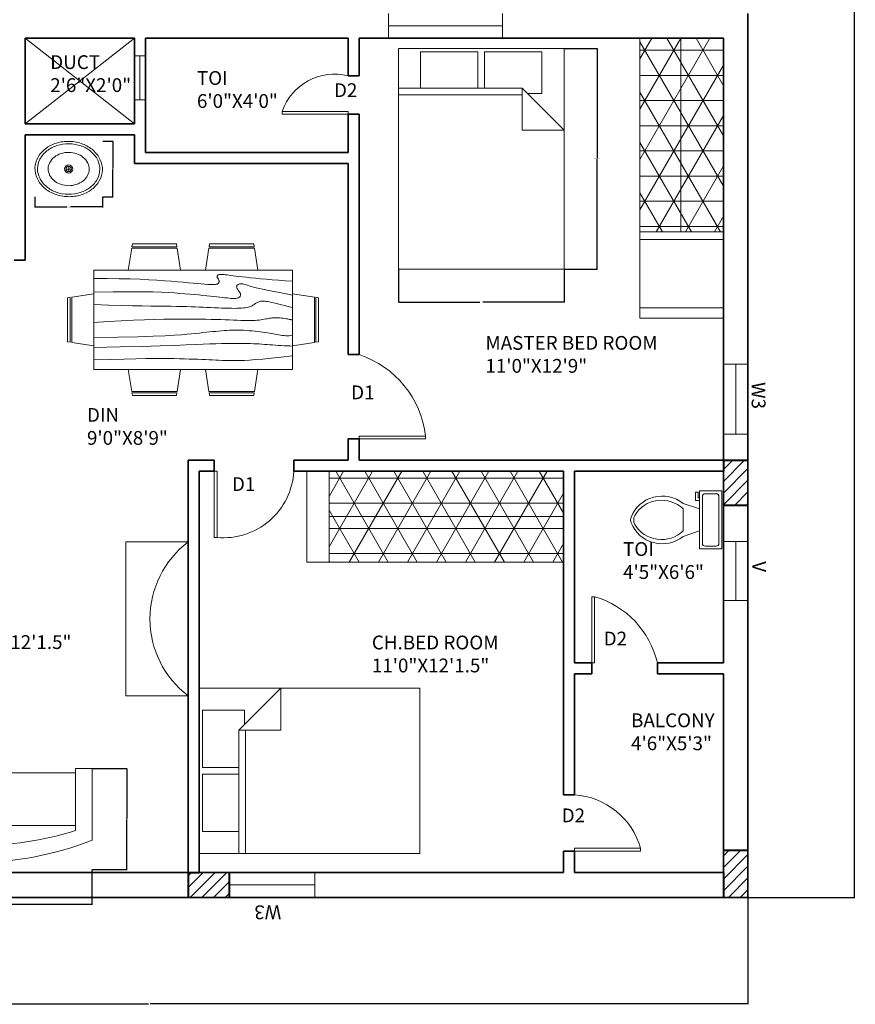
# Model space of a CAD drawing. Units: inches. Extents: x -86 to 2463, y -1058 to 68.
# Tile 2 of 17: x 123 to 426, y -740 to -383. Entities that reach past the tile are written whole.
import ezdxf

# ---------------------------------------------------------------- set-up
doc = ezdxf.new("R2010")
doc.units = ezdxf.units.IN
doc.header["$MEASUREMENT"] = 0
for name, color, linetype, lineweight in [('A-ANNO-DIMS', 2, 'Continuous', 18), ('A-ANNO-TEXT', 7, 'Continuous', 18), ('A-AREA-IDEN', 7, 'Continuous', 18), ('A-COLS', 7, 'Continuous', 40), ('A-COLS-PATT', 252, 'Continuous', 13), ('A-DOOR', 3, 'Continuous', 18), ('A-FLOR-CASE', 8, 'Continuous', 18), ('A-FLOR-CASE-PATT', 252, 'Continuous', 13), ('A-FLOR-FIXT', 9, 'Continuous', 18), ('A-FLOR-OPEN', 8, 'Continuous', 13), ('A-FURN', 8, 'Continuous', 18), ('A-GLAZ', 4, 'Continuous', 18), ('A-WALL', 7, 'Continuous', 35)]:
    doc.layers.add(name, color=color, linetype=linetype, lineweight=lineweight)
doc.styles.get("Standard").update_dxf_attribs({"font": 'arial.ttf'})
doc.dimstyles.get("Standard").update_dxf_attribs({"dimtxt": 0.18, "dimasz": 0.18, "dimexe": 0.18, "dimexo": 0.0625, "dimgap": 0.09, "dimtad": 0, "dimtih": 1, "dimtoh": 1, "dimdec": 4, "dimzin": 0, "dimdsep": 46, "dimtxsty": 'Standard', "dimcen": 0.09, "dimadec": 0, "dimazin": 0, "dimtfac": 1, "dimtdec": 4, "dimtofl": 0, "dimtmove": 0, "dimatfit": 3, "dimfxl": 1, "dimtolj": 1, "dimtzin": 0, "dimarcsym": 0})
pattern_1 = [(45, (-1015.1314, -586.0864), (-2.1213203, 2.1213203), [])]
pattern_2 = [(0, (-1015.131, -586.086), (0, 9.125), []), (60, (-1015.131, -586.086), (-7.90248, 4.5625), []), (120, (-1015.131, -586.086), (-7.90248, -4.5625), [])]

# ---------------------------------------------------------------- blocks, each defined once
blk = doc.blocks.new('Toilet - top')
for p, q in [((9.5, -6), (9.5, -2)), ((-10, -8.5), (-8, -8.5)), ((-10, -9.5), (-10, -8.5)), ((-7, -9.5), (-10, -9.5)), ((-8, -8.5), (-8, -8)), ((-7, -8), (-7, -9.5)), ((-4, -8), (-6, -14)), ((4, -8), (6, -14)), ((4, -14), (-4, -14))]:
    blk.add_line(p, q)
blk.add_lwpolyline([(10.5, -8), (10.5, 0), (-10.5, 0), (-10.5, -8)], close=True)
for points in [[(-9.5, -2), (-9.5, -6)], [(8.5, -1), (-8.5, -1)], [(-8.5, -7), (8.5, -7)]]:
    blk.add_lwpolyline(points)
for centre, radius, start, end in [((-8.62, -1.88), 0.884, 81.8699, 188.1301), ((8.62, -1.88), 0.884, 351.8699, 98.1301), ((-8.62, -6.12), 0.884, 171.8699, 278.1301), ((8.62, -6.12), 0.884, 261.8699, 8.1301), ((3.52, -21.58), 12.17, 141.4691, 247.9714), ((4.2, -21.82), 11.33, 136.3677, 238.9468), ((-3.52, -21.58), 12.17, 292.0284, 38.5307), ((-4.2, -21.82), 11.33, 301.053, 43.6321), ((0, -27.88), 4, 245.7318, 294.2682), ((0, -29), 4, 254.8605, 285.1395)]:
    blk.add_arc(centre, radius, start, end)
blk = doc.blocks.new('Bed - Queen')
for p, q in [((0, -80.00003), (0, 0)), ((0, 0), (59.99999, 0)), ((59.99999, 0), (59.99999, -80.00003)), ((7.99999, -1.2), (28.79998, -1.2)), ((7.99999, -14.4), (7.99999, -1.2)), ((28.79998, -1.2), (28.79998, -14.4)), ((31.19999, -1.2), (51.99999, -1.2)), ((31.19999, -14.4), (31.19999, -1.2)), ((51.99999, -1.2), (51.99999, -16.4)), ((0, -14.4), (44.8, -14.4)), ((44.8, -16.8), (0, -16.8)), ((59.99999, -29.6), (44.8, -14.4)), ((44.8, -14.4), (44.8, -29.6)), ((51.99999, -16.4), (46.79936, -16.4)), ((44.8, -29.6), (59.99999, -29.6)), ((59.99999, -80.00003), (0, -80.00003))]:
    blk.add_line(p, q)
blk = doc.blocks.new('Sink - Oval top')
for p, q in [((-1, 0), (1, 0)), ((0, 1), (0, -1))]:
    blk.add_line(p, q)
for points in [[(-12.23, 0.39, 0.117634), (-11.46, -3.36, 0.104469), (-8.88, -6.8, 0.090016), (-5.08, -9.07, 0.08192), (-0.32, -10.02, 0.08192), (4.49, -9.38, 0.090016), (8.42, -7.36, 0.104469), (11.22, -4.09, 0.117634), (12.23, -0.39, 0.117634), (11.46, 3.36, 0.104469), (8.88, 6.8, 0.090016), (5.08, 9.07, 0.08192), (0.32, 10.02, 0.08192), (-4.49, 9.38, 0.090016), (-8.42, 7.36, 0.104469), (-11.22, 4.09, 0.117634)], [(-11.29, 0.16, 0.118622), (-10.52, -3.25, 0.104678), (-8.07, -6.36, 0.089562), (-4.54, -8.37, 0.081185), (-0.13, -9.15, 0.081185), (4.3, -8.49, 0.089562), (7.89, -6.58, 0.104678), (10.42, -3.55, 0.118622), (11.29, -0.16, 0.118622), (10.52, 3.25, 0.104678), (8.07, 6.36, 0.089562), (4.54, 8.37, 0.081185), (0.13, 9.15, 0.081185), (-4.3, 8.49, 0.089562), (-7.89, 6.58, 0.104678), (-10.42, 3.55, 0.118622)], [(-7.42, 0.08, 0.118283), (-6.91, -2.17, 0.104607), (-5.29, -4.21, 0.089718), (-2.97, -5.53, 0.081436), (-0.07, -6.04, 0.081436), (2.84, -5.59, 0.089718), (5.2, -4.33, 0.104607), (6.86, -2.32, 0.118283), (7.42, -0.08, 0.118283), (6.91, 2.17, 0.104607), (5.29, 4.21, 0.089718), (2.97, 5.53, 0.081436), (0.07, 6.04, 0.081436), (-2.84, 5.59, 0.089718), (-5.2, 4.33, 0.104607), (-6.86, 2.32, 0.118283)]]:
    blk.add_lwpolyline(points, format="xyb", close=True)
for radius in [1.5, 1]:
    blk.add_circle((0, 0), radius)
blk = doc.blocks.new('Sofa - Roundback 7 ft.')
for p, q in [((-12.00002, -32.4421), (-12.00003, -6.5971)), ((11.99997, -32.4421), (11.99998, -6.5971)), ((-36.000027, -34), (-36.000027, -11.4696)), ((-35.999844, -13.3819), (35.9998, -13.3819)), ((35.99998, -34), (35.99998, -11.4696)), ((-36.000027, -32.4421), (35.99998, -32.4421))]:
    blk.add_line(p, q)
for points in [[(-36.000027, -34), (-42.000027, -34), (-42.000027, -8)], [(41.99998, -8), (41.99998, -34), (35.99998, -34)]]:
    blk.add_lwpolyline(points)
for centre, radius, start, end in [((0, -114.25), 114.25, 68.43141, 111.5686), ((-0.00001, -127.1968), 121.1968, 72.72033, 107.2797)]:
    blk.add_arc(centre, radius, start, end)
blk = doc.blocks.new('Dining Set - 36 x 72 in.')
for p, q in [((-22.2343, 26.00059), (-23.4847, 17.99762)), ((-22.2304, 26), (-5.7608, 26)), ((-22, 27.5), (-22.1562, 26.50042)), ((-5.8416, 26.5), (-22.1534, 26.5)), ((-22, 27.5), (-6, 27.5)), ((-5.8437, 26.49966), (-6, 27.5)), ((-4.5152, 17.99762), (-5.7655, 25.99926)), ((5.7657, 26.00059), (4.5153, 17.99762)), ((5.7696, 26), (22.2392, 26)), ((6, 27.5), (5.8438, 26.50042)), ((22.1584, 26.5), (5.8466, 26.5)), ((6, 27.5), (22, 27.5)), ((22.1563, 26.49966), (22, 27.5)), ((23.4848, 17.99762), (22.2345, 25.99926)), ((36, 18), (-36, 18)), ((-36, 18), (-36, -18)), ((36, -18), (36, 18)), ((-45.5, 8), (-44.5004, 8.15617)), ((-45.5, 8), (-45.5, -8)), ((-44.5, -8.15843), (-44.5, 8.15338)), ((-44.0006, 8.23428), (-35.9976, 9.48474)), ((-44, 8.23041), (-44, -8.23915)), ((44.0006, 8.23428), (35.9976, 9.48474)), ((44, 8.23041), (44, -8.23915)), ((44.5, -8.15843), (44.5, 8.15338)), ((45.5, 8), (44.5005, 8.15617)), ((45.5, 8), (45.5, -8)), ((-44.4997, -8.15631), (-45.5, -8)), ((-35.9976, -9.48476), (-43.9993, -8.2345)), ((35.9976, -9.48476), (43.9993, -8.2345)), ((44.4997, -8.15631), (45.5, -8)), ((-36, -18), (36, -18)), ((-22.2343, -26.0006), (-23.4847, -17.99762)), ((-4.5152, -17.99762), (-5.7655, -25.99928)), ((5.7657, -26.0006), (4.5153, -17.99762)), ((23.4848, -17.99762), (22.2345, -25.99928)), ((-22.2304, -26), (-5.7608, -26)), ((-22, -27.5), (-22.1562, -26.50044)), ((-5.8416, -26.5), (-22.1534, -26.5)), ((-22, -27.5), (-6, -27.5)), ((-5.8437, -26.49967), (-6, -27.5)), ((5.7696, -26), (22.2392, -26)), ((6, -27.5), (5.8438, -26.50044)), ((22.1584, -26.5), (5.8466, -26.5)), ((6, -27.5), (22, -27.5)), ((22.1563, -26.49967), (22, -27.5))]:
    blk.add_line(p, q)
for points in [[(-36, 15), (-31.1772, 14.97754), (-26.8079, 14.91406), (-22.8538, 14.81543), (-19.276, 14.6875), (-16.0362, 14.53613), (-13.0957, 14.36718), (-10.4159, 14.18652), (-7.9583, 14), (-5.6904, 13.81315), (-3.6035, 13.63021), (-1.6954, 13.45508), (0.0365, 13.29166), (1.5945, 13.14388), (2.9811, 13.01562), (4.1988, 12.9108), (5.25, 12.83333), (6.1393, 12.78613), (6.8802, 12.76823), (7.4883, 12.77767), (7.9792, 12.8125), (8.3685, 12.87077), (8.6719, 12.95052), (8.9049, 13.0498), (9.0833, 13.16666), (9.2205, 13.29899), (9.3216, 13.44401), (9.3895, 13.59879), (9.4271, 13.76041), (9.4373, 13.92594), (9.4232, 14.09245), (9.3875, 14.257), (9.3333, 14.41666), (9.2638, 14.56917), (9.1836, 14.71484), (9.0975, 14.85465), (9.0104, 14.98958), (8.9272, 15.1206), (8.8529, 15.2487), (8.7922, 15.37483), (8.75, 15.5), (8.7305, 15.62467), (8.7344, 15.74739), (8.7617, 15.86621), (8.8125, 15.97916), (8.8867, 16.08431), (8.9844, 16.17968), (9.1055, 16.26334), (9.25, 16.33333), (9.4189, 16.38802), (9.6172, 16.42708), (9.8506, 16.45052), (10.125, 16.45833), (10.4463, 16.45052), (10.8203, 16.42708), (11.2529, 16.38802), (11.75, 16.33333), (12.3184, 16.26318), (12.9694, 16.17838), (13.7151, 16.07991), (14.5677, 15.96875), (15.5395, 15.84586), (16.6426, 15.71224), (17.8893, 15.56884), (19.2917, 15.41666), (20.859, 15.25667), (22.5879, 15.08984), (24.4721, 14.91715), (26.5052, 14.73958), (28.6809, 14.5581), (30.9929, 14.3737), (33.4347, 14.18733), (36, 14)], [(-36, 10), (-28.9766, 10.14274), (-23.1725, 10.20442), (-18.4241, 10.19775), (-14.5677, 10.13541), (-11.4399, 10.03011), (-8.877, 9.89453), (-6.7154, 9.74137), (-4.7917, 9.58333), (-2.9698, 9.43082), (-1.2246, 9.28515), (0.4415, 9.14534), (2.026, 9.01041), (3.5266, 8.87939), (4.9408, 8.7513), (6.266, 8.62516), (7.5, 8.5), (8.6411, 8.37549), (9.6914, 8.2539), (10.6538, 8.13818), (11.5312, 8.03125), (12.3267, 7.93603), (13.043, 7.85547), (13.6831, 7.79248), (14.25, 7.75), (14.7471, 7.7303), (15.1797, 7.73307), (15.5537, 7.75732), (15.875, 7.80208), (16.1494, 7.86637), (16.3828, 7.94922), (16.5811, 8.04964), (16.75, 8.16666), (16.8944, 8.29915), (17.0143, 8.44531), (17.1089, 8.60319), (17.1771, 8.77083), (17.218, 8.94629), (17.2305, 9.1276), (17.2137, 9.31282), (17.1667, 9.5), (17.0895, 9.6875), (16.987, 9.875), (16.8649, 10.0625), (16.7292, 10.25), (16.5856, 10.4375), (16.4401, 10.625), (16.2985, 10.8125), (16.1667, 11), (16.05, 11.18733), (15.9518, 11.3737), (15.8752, 11.5581), (15.8229, 11.73958), (15.798, 11.91715), (15.8034, 12.08984), (15.842, 12.25667), (15.9167, 12.41666), (16.0295, 12.56836), (16.1784, 12.70833), (16.3605, 12.83268), (16.5729, 12.9375), (16.8127, 13.01888), (17.0768, 13.07291), (17.3625, 13.0957), (17.6667, 13.08333), (17.9894, 13.03312), (18.3418, 12.94726), (18.7382, 12.82918), (19.1927, 12.68229), (19.7195, 12.51001), (20.3327, 12.31575), (21.0465, 12.10294), (21.875, 11.875), (22.8357, 11.63354), (23.959, 11.37304), (25.2786, 11.08618), (26.8282, 10.76562), (28.6414, 10.40405), (30.752, 9.99414), (33.1936, 9.52856), (36, 9)], [(-36, 5.5), (-30.7157, 5.3348), (-26.069, 5.20963), (-21.9946, 5.11767), (-18.4271, 5.05208), (-15.3009, 5.00602), (-12.5508, 4.97265), (-10.1112, 4.94515), (-7.9167, 4.91666), (-5.909, 4.88167), (-4.0586, 4.83984), (-2.3429, 4.79215), (-0.7396, 4.73958), (0.7739, 4.6831), (2.22, 4.6237), (3.6213, 4.56233), (5, 4.5), (6.373, 4.43782), (7.7344, 4.3776), (9.0723, 4.32129), (10.375, 4.27083), (11.6309, 4.22819), (12.8281, 4.19531), (13.9551, 4.17415), (15, 4.16666), (15.954, 4.17448), (16.819, 4.19791), (17.6001, 4.23698), (18.3021, 4.29166), (18.9299, 4.36198), (19.4883, 4.44791), (19.9823, 4.54948), (20.4167, 4.66666), (20.7969, 4.79899), (21.1302, 4.94401), (21.4245, 5.09879), (21.6875, 5.26041), (21.9271, 5.42594), (22.1511, 5.59245), (22.3672, 5.757), (22.5834, 5.91666), (22.8065, 6.06868), (23.0404, 6.21093), (23.2879, 6.34147), (23.5521, 6.45833), (23.8358, 6.55957), (24.142, 6.64323), (24.4735, 6.70735), (24.8334, 6.75), (25.2235, 6.76969), (25.642, 6.76692), (26.0858, 6.74267), (26.5521, 6.69791), (27.0379, 6.63362), (27.5404, 6.55078), (28.0565, 6.45036), (28.5834, 6.33333), (29.1242, 6.19987), (29.7071, 6.04687), (30.3661, 5.87044), (31.1354, 5.66666), (32.0493, 5.43164), (33.142, 5.16146), (34.4475, 4.85221), (36, 4.5)], [(-36, -1), (-30.7915, -0.6591), (-26.0195, -0.38216), (-21.6519, -0.16284), (-17.6563, 0.00521), (-14.0005, 0.12833), (-10.6523, 0.21289), (-7.5796, 0.26522), (-4.75, 0.29166), (-2.134, 0.29793), (0.2878, 0.28711), (2.5317, 0.26163), (4.6146, 0.22396), (6.5529, 0.17651), (8.3633, 0.12174), (10.0623, 0.06209), (11.6667, 0), (13.1899, -0.06201), (14.6341, -0.1211), (15.9982, -0.17432), (17.2813, -0.21875), (18.4823, -0.25147), (19.6003, -0.26953), (20.6343, -0.27002), (21.5834, -0.25), (22.4481, -0.20768), (23.2357, -0.14584), (23.9549, -0.06836), (24.6146, 0.02083), (25.2235, 0.11784), (25.7904, 0.21875), (26.3241, 0.31966), (26.8334, 0.41666), (27.3265, 0.50618), (27.8099, 0.58593), (28.2894, 0.65397), (28.7709, 0.70833), (29.2601, 0.74707), (29.763, 0.76823), (30.2855, 0.76985), (30.8334, 0.75), (31.4088, 0.70784), (31.9994, 0.64713), (32.589, 0.57275), (33.1615, 0.48958), (33.7008, 0.4025), (34.1908, 0.3164), (34.6153, 0.23616), (34.9584, 0.16666), (35.2099, 0.11165), (35.3848, 0.07031), (35.504, 0.04069), (35.5886, 0.02083), (35.6594, 0.00879), (35.7377, 0.0026), (35.8442, 0.00032), (36, 0)], [(-36, -6.5), (-27.1843, -6.31267), (-20.084, -6.1263), (-14.469, -5.9419), (-10.1094, -5.76042), (-6.7752, -5.58285), (-4.2363, -5.41016), (-2.2629, -5.24333), (-0.625, -5.08334), (0.8708, -4.93099), (2.2715, -4.78646), (3.5872, -4.64974), (4.8281, -4.52084), (6.0046, -4.39974), (7.127, -4.28646), (8.2053, -4.18099), (9.25, -4.08334), (10.2705, -3.99382), (11.2734, -3.91407), (12.2647, -3.84603), (13.25, -3.79167), (14.2354, -3.75293), (15.2266, -3.73177), (16.2295, -3.73015), (17.25, -3.75), (18.2912, -3.79248), (19.3451, -3.85547), (20.4009, -3.93604), (21.4479, -4.03125), (22.4754, -4.13819), (23.4727, -4.25391), (24.4289, -4.37549), (25.3334, -4.5), (26.1785, -4.62492), (26.9694, -4.74935), (27.7145, -4.87281), (28.4219, -4.99479), (29.1, -5.11483), (29.7572, -5.23242), (30.4016, -5.34709), (31.0417, -5.45834), (31.6837, -5.56437), (32.3262, -5.65821), (32.9658, -5.73153), (33.599, -5.77604), (34.2224, -5.78345), (34.8327, -5.74545), (35.4264, -5.65373), (36, -5.5)], [(-36, -10), (-26.4022, -9.81299), (-18.4675, -9.62891), (-11.9839, -9.45069), (-6.7396, -9.28125), (-2.5226, -9.12354), (0.8789, -8.98047), (3.6769, -8.85498), (6.0833, -8.75), (8.2767, -8.66765), (10.3021, -8.60677), (12.1712, -8.56543), (13.8958, -8.54167), (15.4876, -8.53353), (16.9583, -8.53907), (18.3197, -8.55632), (19.5834, -8.58334), (20.7616, -8.61841), (21.8685, -8.66081), (22.9188, -8.71004), (23.9271, -8.76563), (24.9081, -8.82707), (25.8763, -8.89388), (26.8465, -8.96558), (27.8334, -9.04167), (28.8474, -9.12118), (29.8828, -9.20117), (30.93, -9.27824), (31.9792, -9.34896), (33.0205, -9.40991), (34.0443, -9.45768), (35.0407, -9.48885), (36, -9.5)], [(-36, -14.5), (-30.0881, -14.33513), (-25.0332, -14.21224), (-20.7312, -14.12647), (-17.0781, -14.07292), (-13.97, -14.04671), (-11.3027, -14.04297), (-8.9724, -14.05681), (-6.875, -14.08334), (-4.9224, -14.11833), (-3.0905, -14.16016), (-1.3709, -14.20785), (0.2448, -14.26042), (1.7647, -14.3169), (3.1973, -14.3763), (4.5507, -14.43767), (5.8333, -14.5), (7.0554, -14.5621), (8.235, -14.62175), (9.3922, -14.67652), (10.5469, -14.72396), (11.7192, -14.76164), (12.929, -14.78711), (14.1965, -14.79794), (15.5417, -14.79167), (16.9933, -14.76424), (18.6152, -14.70508), (20.4804, -14.60197), (22.6615, -14.44271), (25.2312, -14.21509), (28.2624, -13.9069), (31.8277, -13.50594), (36, -13)]]:
    blk.add_lwpolyline(points)
blk = doc.blocks.new('DOOR-LEAF-24IN')
for p, q in [((0, 0), (0, 24)), ((0, 24), (1, 24)), ((1, 24), (1, 0)), ((1, 0), (0, 0))]:
    blk.add_line(p, q)
blk = doc.blocks.new('*D12')
at = {"layer": 'A-ANNO-DIMS', "color": 0, "lineweight": -2, "transparency": 16777216}
for p, q in [((320.14, -393.76), (332.26, -393.76)), ((332.08, -393.94), (332.08, -433.57)), ((332.08, -473.58), (332.08, -433.95)), ((320.14, -473.76), (332.26, -473.76))]:
    blk.add_line(p, q, dxfattribs=at)
at = {"layer": 'A-ANNO-DIMS', "color": 0, "transparency": 16777216}
for points in [[(332.05, -393.94), (332.11, -393.94), (332.08, -393.76)], [(332.05, -473.58), (332.11, -473.58), (332.08, -473.76)]]:
    blk.add_solid(points, dxfattribs=at)
at = {"layer": 'Defpoints', "color": 0, "transparency": 16777216}
for p in [(320.08, -393.76), (332.08, -393.76), (320.08, -473.76)]:
    blk.add_point(p, dxfattribs=at)
at = {"layer": 'A-ANNO-DIMS', "color": 0, "transparency": 16777216, "insert": (332.08, -433.76), "char_height": 0.18, "attachment_point": 5}
blk.add_mtext('\\A1;QUEEN BED 80 TYP.', dxfattribs=at)
blk = doc.blocks.new('*D13')
at = {"layer": 'A-ANNO-DIMS', "color": 0, "lineweight": -2, "transparency": 16777216}
for p, q in [((260.08, -473.82), (260.08, -485.94)), ((320.08, -473.82), (320.08, -485.94)), ((260.26, -485.76), (289.55, -485.76)), ((319.9, -485.76), (290.61, -485.76))]:
    blk.add_line(p, q, dxfattribs=at)
at = {"layer": 'A-ANNO-DIMS', "color": 0, "transparency": 16777216}
for points in [[(260.26, -485.73), (260.26, -485.79), (260.08, -485.76)], [(319.9, -485.73), (319.9, -485.79), (320.08, -485.76)]]:
    blk.add_solid(points, dxfattribs=at)
at = {"layer": 'Defpoints', "color": 0, "transparency": 16777216}
for p in [(260.08, -473.76), (320.08, -473.76), (320.08, -485.76)]:
    blk.add_point(p, dxfattribs=at)
at = {"layer": 'A-ANNO-DIMS', "color": 0, "transparency": 16777216, "insert": (290.08, -485.76), "char_height": 0.18, "attachment_point": 5}
blk.add_mtext('\\A1;60 TYP.', dxfattribs=at)
blk = doc.blocks.new('*D20')
at = {"layer": 'A-ANNO-DIMS', "color": 0, "lineweight": -2, "transparency": 16777216}
for p, q in [((128.24, -447.63), (128.24, -451.43)), ((152.8, -447.63), (152.8, -451.43)), ((128.42, -451.25), (139.89, -451.25)), ((152.62, -451.25), (141.15, -451.25))]:
    blk.add_line(p, q, dxfattribs=at)
at = {"layer": 'A-ANNO-DIMS', "color": 0, "transparency": 16777216}
for points in [[(128.42, -451.22), (128.42, -451.28), (128.24, -451.25)], [(152.62, -451.22), (152.62, -451.28), (152.8, -451.25)]]:
    blk.add_solid(points, dxfattribs=at)
at = {"layer": 'Defpoints', "color": 0, "transparency": 16777216}
for p in [(128.24, -447.57), (152.8, -447.57), (152.8, -451.25)]:
    blk.add_point(p, dxfattribs=at)
at = {"layer": 'A-ANNO-DIMS', "color": 0, "transparency": 16777216, "insert": (140.52, -451.25), "char_height": 0.18, "attachment_point": 5}
blk.add_mtext('\\A1;BASIN 25', dxfattribs=at)
blk = doc.blocks.new('*D21')
at = {"layer": 'A-ANNO-DIMS', "color": 0, "lineweight": -2, "transparency": 16777216}
for p, q in [((152.86, -427.44), (156.66, -427.44)), ((156.48, -427.62), (156.48, -437.32)), ((156.48, -447.39), (156.48, -437.69)), ((152.86, -447.57), (156.66, -447.57))]:
    blk.add_line(p, q, dxfattribs=at)
at = {"layer": 'A-ANNO-DIMS', "color": 0, "transparency": 16777216}
for points in [[(156.45, -427.62), (156.51, -427.62), (156.48, -427.44)], [(156.45, -447.39), (156.51, -447.39), (156.48, -447.57)]]:
    blk.add_solid(points, dxfattribs=at)
at = {"layer": 'Defpoints', "color": 0, "transparency": 16777216}
for p in [(152.8, -427.44), (156.48, -427.44), (152.8, -447.57)]:
    blk.add_point(p, dxfattribs=at)
at = {"layer": 'A-ANNO-DIMS', "color": 0, "transparency": 16777216, "insert": (156.48, -437.5), "char_height": 0.18, "attachment_point": 5}
blk.add_mtext('\\A1;20', dxfattribs=at)
blk = doc.blocks.new('*D26')
at = {"layer": 'A-ANNO-DIMS', "color": 0, "lineweight": -2, "transparency": 16777216}
for p, q in [((64.97, -691.61), (64.97, -704.32)), ((148.97, -691.61), (148.97, -704.32)), ((65.15, -704.14), (106.07, -704.14)), ((148.79, -704.14), (107.88, -704.14))]:
    blk.add_line(p, q, dxfattribs=at)
at = {"layer": 'A-ANNO-DIMS', "color": 0, "transparency": 16777216}
for points in [[(65.15, -704.11), (65.15, -704.17), (64.97, -704.14)], [(148.79, -704.11), (148.79, -704.17), (148.97, -704.14)]]:
    blk.add_solid(points, dxfattribs=at)
at = {"layer": 'Defpoints', "color": 0, "transparency": 16777216}
for p in [(64.97, -691.54), (148.97, -691.54), (64.97, -704.14)]:
    blk.add_point(p, dxfattribs=at)
at = {"layer": 'A-ANNO-DIMS', "color": 0, "transparency": 16777216, "insert": (106.97, -704.14), "char_height": 0.18, "attachment_point": 5}
blk.add_mtext('\\A1;SOFA 84 TYP.', dxfattribs=at)
blk = doc.blocks.new('*D27')
at = {"layer": 'A-ANNO-DIMS', "color": 0, "lineweight": -2, "transparency": 16777216}
for p, q in [((149.04, -654.88), (161.75, -654.88)), ((161.57, -655.06), (161.57, -673.03)), ((161.57, -691.36), (161.57, -673.39)), ((149.04, -691.54), (161.75, -691.54))]:
    blk.add_line(p, q, dxfattribs=at)
at = {"layer": 'A-ANNO-DIMS', "color": 0, "transparency": 16777216}
for points in [[(161.54, -655.06), (161.6, -655.06), (161.57, -654.88)], [(161.54, -691.36), (161.6, -691.36), (161.57, -691.54)]]:
    blk.add_solid(points, dxfattribs=at)
at = {"layer": 'Defpoints', "color": 0, "transparency": 16777216}
for p in [(148.97, -654.88), (148.97, -691.54), (161.57, -691.54)]:
    blk.add_point(p, dxfattribs=at)
at = {"layer": 'A-ANNO-DIMS', "color": 0, "transparency": 16777216, "insert": (161.57, -673.21), "char_height": 0.18, "attachment_point": 5}
blk.add_mtext('\\A1;37 TYP.', dxfattribs=at)
blk = doc.blocks.new('*D30')
at = {"layer": 'A-ANNO-DIMS', "color": 0, "lineweight": -2, "transparency": 16777216}
for p, q in [((-47.24, -701.67), (-47.24, -740.38)), ((386.76, -701.67), (386.76, -740.38)), ((-47.06, -740.2), (169.47, -740.2)), ((386.58, -740.2), (170.05, -740.2))]:
    blk.add_line(p, q, dxfattribs=at)
at = {"layer": 'A-ANNO-DIMS', "color": 0, "transparency": 16777216}
for points in [[(-47.06, -740.17), (-47.06, -740.23), (-47.24, -740.2)], [(386.58, -740.17), (386.58, -740.23), (386.76, -740.2)]]:
    blk.add_solid(points, dxfattribs=at)
at = {"layer": 'Defpoints', "color": 0, "transparency": 16777216}
for p in [(-47.24, -701.6), (386.76, -701.6), (386.76, -740.2)]:
    blk.add_point(p, dxfattribs=at)
at = {"layer": 'A-ANNO-DIMS', "color": 0, "transparency": 16777216, "insert": (169.76, -740.2), "char_height": 0.18, "attachment_point": 5}
blk.add_mtext('\\A1;434', dxfattribs=at)
blk = doc.blocks.new('*D31')
at = {"layer": 'A-ANNO-DIMS', "color": 0, "lineweight": -2, "transparency": 16777216}
for p, q in [((386.82, 28.9), (425.54, 28.9)), ((425.36, 28.72), (425.36, -336.17)), ((425.36, -701.42), (425.36, -336.54)), ((386.82, -701.6), (425.54, -701.6))]:
    blk.add_line(p, q, dxfattribs=at)
at = {"layer": 'A-ANNO-DIMS', "color": 0, "transparency": 16777216}
for points in [[(425.33, 28.72), (425.39, 28.72), (425.36, 28.9)], [(425.33, -701.42), (425.39, -701.42), (425.36, -701.6)]]:
    blk.add_solid(points, dxfattribs=at)
at = {"layer": 'Defpoints', "color": 0, "transparency": 16777216}
for p in [(386.76, 28.9), (425.36, 28.9), (386.76, -701.6)]:
    blk.add_point(p, dxfattribs=at)
at = {"layer": 'A-ANNO-DIMS', "color": 0, "transparency": 16777216, "insert": (425.36, -336.35), "char_height": 0.18, "attachment_point": 5}
blk.add_mtext('\\A1;730.5', dxfattribs=at)

msp = doc.modelspace()

# ---------------------------------------------------------------- hatches: boundary and pattern name
at = {"layer": 'A-COLS-PATT'}
h = msp.add_hatch(dxfattribs=at)
h.set_pattern_fill('ANSI31', color=256, scale=24)
h.set_pattern_definition(pattern_1)
h.paths.add_polyline_path([(386.761, -543.104), (377.846, -543.104), (377.846, -547.104), (377.846, -559.337), (386.761, -559.337)])
h.paths.add_polyline_path([(24.761, -547.104), (24.761, -543.104), (24.761, -538.166), (15.761, -538.166), (15.761, -559.72), (24.761, -559.72)])
h = msp.add_hatch(dxfattribs=at)
h.set_pattern_fill('ANSI31', color=256, scale=24)
h.set_pattern_definition(pattern_1)
h.paths.add_polyline_path([(24.761, -676.336), (15.761, -676.336), (15.761, -701.604), (24.761, -701.604), (24.761, -692.604)])
h.paths.add_polyline_path([(198.701, -692.604), (187.846, -692.604), (183.846, -692.604), (183.846, -701.604), (198.701, -701.604)])
h.paths.add_polyline_path([(386.761, -684.448), (377.846, -684.448), (377.846, -692.604), (377.846, -701.604), (386.761, -701.604)])
at = {"layer": 'A-FLOR-CASE-PATT'}
h = msp.add_hatch(dxfattribs=at)
h.set_pattern_fill('NET3', color=256, scale=73)
h.set_pattern_definition(pattern_2)
h.paths.add_polyline_path([(362.202, 19.896), (346.643, 19.896), (346.643, -48.262), (362.202, -48.262)])
h.paths.add_polyline_path([(377.761, 19.896), (362.202, 19.896), (362.202, -48.262), (377.761, -48.262)])
h.paths.add_polyline_path([(362.455, -390.104), (347.604, -390.104), (347.604, -460.245), (362.455, -460.245)])
h.paths.add_polyline_path([(377.846, -390.104), (362.455, -390.104), (362.455, -460.245), (377.846, -460.245), (377.846, -425.104), (377.846, -421.104)])
h = msp.add_hatch(dxfattribs=at)
h.set_pattern_fill('NET3', color=256, scale=73)
h.set_pattern_definition(pattern_2)
h.paths.add_polyline_path([(319.761, -145.104), (227.044, -145.104), (227.044, -157.07), (319.761, -157.07)])
h.paths.add_polyline_path([(319.761, -157.07), (227.044, -157.07), (227.044, -169.036), (319.761, -169.036)])
h.paths.add_polyline_path([(319.846, -547.104), (234.906, -547.104), (234.906, -563.554), (319.846, -563.554)])
h.paths.add_polyline_path([(319.846, -563.554), (234.906, -563.554), (234.906, -580.004), (319.846, -580.004)])

# ---------------------------------------------------------------- linework, layer by layer
at = {"layer": 'A-COLS'}
for p, q in [((377.846, -543.104), (386.761, -543.104)), ((377.846, -543.104), (377.846, -547.104)), ((377.846, -559.337), (386.761, -559.337)), ((377.846, -684.448), (386.761, -684.448)), ((183.846, -692.604), (187.846, -692.604)), ((183.846, -692.604), (183.846, -701.604)), ((198.701, -692.604), (198.701, -701.604)), ((377.846, -692.604), (377.846, -701.604))]:
    msp.add_line(p, q, dxfattribs=at)
at = {"layer": 'A-DOOR'}
for centre, radius, start, end in [((236.952, -423.345), 20.241, 76.00679, 160.72316), ((234.855, -538.265), 35.209, 6.38342, 71.81059), ((196.648, -545.684), 25.53, 264.68315, 356.81017), ((322.213, -623.866), 32.521, 12.90257, 74.00492), ((322.101, -691.123), 26.766, 15.87539, 86.26146)]:
    msp.add_arc(centre, radius, start, end, dxfattribs=at)
at = {"layer": 'A-FLOR-CASE'}
for p, q in [((347.604, -491.608), (347.604, -390.104)), ((362.455, -390.104), (362.455, -460.245)), ((347.604, -460.245), (377.846, -460.245)), ((347.604, -463.001), (377.846, -463.001)), ((347.604, -487.822), (377.846, -487.822)), ((377.846, -491.608), (347.604, -491.608)), ((226.835, -547.104), (226.835, -580.004)), ((234.906, -547.104), (234.906, -580.004)), ((234.906, -563.554), (319.846, -563.554)), ((183.846, -572.736), (161.177, -572.736)), ((161.177, -572.736), (161.177, -628.527)), ((226.835, -580.004), (319.846, -580.004)), ((161.177, -628.527), (183.846, -628.527))]:
    msp.add_line(p, q, dxfattribs=at)
msp.add_arc((204.965, -600.632), 34.988, 127.12835, 232.87165, dxfattribs=at)
at = {"layer": 'A-FLOR-OPEN'}
for p, q in [((124.761, -390.104), (164.346, -421.104)), ((124.761, -421.104), (164.346, -390.104))]:
    msp.add_line(p, q, dxfattribs=at)
at = {"layer": 'A-GLAZ'}
for p, q in [((256.416, -390.104), (256.416, -381.104)), ((297.782, -390.104), (297.782, -381.104)), ((257.59, -385.604), (256.416, -385.604)), ((257.59, -385.604), (297.782, -385.604)), ((164.346, -396.407), (168.346, -396.407)), ((166.346, -396.407), (166.346, -412.367)), ((164.346, -412.367), (168.346, -412.367)), ((377.846, -508.264), (386.761, -508.264)), ((382.303, -533.626), (382.303, -508.264)), ((377.846, -533.626), (386.761, -533.626)), ((377.846, -572.519), (386.761, -572.519)), ((382.303, -572.519), (382.303, -593.945)), ((377.846, -593.945), (386.761, -593.945)), ((229.726, -692.604), (229.726, -701.604)), ((198.701, -697.104), (229.726, -697.104))]:
    msp.add_line(p, q, dxfattribs=at)
at = {"layer": 'A-WALL'}
for p, q in [((386.761, -390.104), (386.761, -381.104)), ((124.761, -390.104), (124.761, -421.104)), ((164.346, -390.104), (124.761, -390.104)), ((164.346, -390.104), (164.346, -421.104)), ((168.346, -390.104), (168.346, -421.104)), ((241.846, -390.104), (168.346, -390.104)), ((241.846, -390.104), (241.846, -403.705)), ((377.846, -390.104), (245.846, -390.104)), ((245.846, -390.104), (245.846, -403.705)), ((377.846, -390.104), (377.846, -421.104)), ((386.761, -390.104), (386.761, -701.604)), ((241.846, -403.705), (245.846, -403.705)), ((241.846, -417.663), (245.846, -417.663)), ((241.846, -417.663), (241.846, -421.104)), ((245.846, -417.663), (245.846, -421.104)), ((164.346, -421.104), (124.761, -421.104)), ((168.346, -421.104), (168.346, -431.539)), ((241.846, -425.104), (241.846, -421.104)), ((245.846, -419.383), (245.846, -425.104)), ((377.846, -421.104), (377.846, -425.104)), ((124.761, -425.104), (124.761, -470.557)), ((164.346, -425.104), (124.761, -425.104)), ((164.346, -425.104), (164.346, -431.539)), ((241.846, -425.104), (241.846, -431.539)), ((245.846, -425.104), (245.846, -504.815)), ((377.846, -425.104), (377.846, -543.104)), ((164.346, -431.539), (164.346, -435.539)), ((168.346, -431.539), (241.846, -431.539)), ((164.346, -435.539), (241.846, -435.539)), ((241.846, -435.539), (241.846, -504.815)), ((120.761, -470.557), (124.761, -470.557)), ((241.846, -504.815), (245.846, -504.815)), ((241.846, -535.35), (245.846, -535.35)), ((241.846, -535.35), (241.846, -543.104)), ((245.846, -535.35), (245.846, -543.104)), ((183.846, -543.104), (183.846, -692.604)), ((193.283, -543.104), (183.846, -543.104)), ((193.283, -547.104), (193.283, -543.104)), ((241.846, -543.104), (222.139, -543.104)), ((222.139, -547.104), (222.139, -543.104)), ((377.846, -543.104), (245.846, -543.104)), ((187.846, -547.104), (187.846, -692.604)), ((193.283, -547.104), (187.846, -547.104)), ((319.846, -547.104), (222.139, -547.104)), ((319.846, -547.104), (319.846, -664.414)), ((377.846, -547.104), (323.846, -547.104)), ((323.846, -547.104), (323.846, -616.604)), ((377.846, -547.104), (377.846, -616.604)), ((330.174, -616.604), (323.846, -616.604)), ((330.174, -620.604), (330.174, -616.604)), ((377.846, -616.604), (353.912, -616.604)), ((353.912, -620.604), (353.912, -616.604)), ((330.174, -620.604), (323.846, -620.604)), ((323.846, -620.604), (323.846, -664.414)), ((377.846, -620.604), (353.912, -620.604)), ((377.846, -620.604), (377.846, -692.604)), ((319.846, -664.414), (323.846, -664.414)), ((319.846, -684.802), (323.846, -684.802)), ((319.846, -684.802), (319.846, -692.604)), ((323.846, -684.802), (323.846, -692.604)), ((183.846, -692.604), (24.761, -692.604)), ((319.846, -692.604), (187.846, -692.604)), ((377.846, -692.604), (323.846, -692.604)), ((386.761, -701.604), (15.761, -701.604))]:
    msp.add_line(p, q, dxfattribs=at)

# ---------------------------------------------------------------- block references
at = {"layer": 'A-DOOR'}
for p, rotation in [((217.846, -416.663), 270.0000000000001), ((245.846, -534.35), 270.0000000000001), ((194.283, -547.104), 180), ((331.174, -592.604), 180), ((323.846, -683.802), 270.0000000000001)]:
    msp.add_blockref('DOOR-LEAF-24IN', p, dxfattribs=dict(at, rotation=rotation))
at = {"layer": 'A-FLOR-FIXT'}
msp.add_blockref('Sink - Oval top', (140.52, -437.503), dxfattribs=at)
at = {"layer": 'A-FLOR-FIXT', "rotation": 270}
msp.add_blockref('Toilet - top', (377.231, -564.73), dxfattribs=at)
at = {"layer": 'A-FURN'}
for name, p in [('Bed - Queen', (260.077, -393.76)), ('Dining Set - 36 x 72 in.', (185.611, -492.185))]:
    msp.add_blockref(name, p, dxfattribs=at)
for name, p, rotation in [('Bed - Queen', (187.846, -685.729), 90), ('Sofa - Roundback 7 ft.', (106.975, -688.878), 180)]:
    msp.add_blockref(name, p, dxfattribs=dict(at, rotation=rotation))

# ---------------------------------------------------------------- texts
at = {"layer": 'A-ANNO-TEXT', "char_height": 5, "attachment_point": 1}
for s, width, insert in [('D2', 8.29936, (236.693, -406.413)), ('D1', 12.22352, (242.92, -515.993)), ('D1', 7.87641, (199.706, -549.24)), ('D2', 9.73341, (334.463, -605.263)), ('D2', 13.40627, (319.237, -669.38))]:
    msp.add_mtext_dynamic_manual_height_columns(s, width=width, gutter_width=25, heights=[0], dxfattribs=dict(at, insert=insert))
for s, width, insert, rotation in [('W3', 13.02181, (393.098, -514.751), 270), ('V', 8.04337, (393.348, -579.713), 270), ('W3', 15.84226, (217.573, -709.53), 180)]:
    msp.add_mtext_dynamic_manual_height_columns(s, width=width, gutter_width=25, heights=[0], dxfattribs=dict(at, insert=insert, rotation=rotation))
at = {"layer": 'A-AREA-IDEN', "char_height": 5, "attachment_point": 1}
for s, width, insert in [('DUCT\\P2\'6"X2\'0"', 29.31073, (133.831, -396.245)), ('TOI\\P6\'0"X4\'0"', 24.13948, (187.015, -402.008)), ('MASTER BED ROOM\\P11\'0"X12\'9"', 128.16745, (291.582, -498.047)), ('DIN\\P9\'0"X8\'9"', 33.48911, (147.153, -524.171)), ('TOI\\P4\'5"X6\'6"', 37.88678, (341.48, -572.801)), ('HALL\\P13\'3"X12\'1.5"', 75.18459, (98.956, -598.214)), ('CH.BED ROOM\\P11\'0"X12\'1.5"', 110.29173, (250.42, -606.687)), ('BALCONY\\P4\'6"X5\'3"', 41.28173, (344.379, -634.906))]:
    msp.add_mtext_dynamic_manual_height_columns(s, width=width, gutter_width=25, heights=[0], dxfattribs=dict(at, insert=insert))

# ---------------------------------------------------------------- dimensions: what is measured, and where the dimension line sits
at = {"layer": 'A-ANNO-DIMS'}
for base, p1, p2, override, picture, middle in [((425.361, 28.896), (386.761, -701.604), (386.761, 28.896), {"dimdec": 1, "dimlfac": 1, "dimrnd": 0, "dimzin": 0, "dimdsep": 46, "dimlunit": 2}, '*D31', (425.361, -336.354)), ((156.478, -427.435), (152.796, -447.572), (152.796, -427.435), {"dimdec": 0, "dimlfac": 1, "dimrnd": 0, "dimzin": 0, "dimdsep": 46, "dimlunit": 2}, '*D21', (156.478, -437.503))]:
    dim = msp.add_linear_dim(base=base, p1=p1, p2=p2, angle=90, dimstyle='Standard', override=override, dxfattribs=at)
    dim.commit()
    dim.dimension.update_dxf_attribs({"geometry": picture, "text_midpoint": middle})
for base, p1, p2, angle, text, picture, middle in [((332.077, -393.76), (320.077, -473.76), (320.077, -393.76), 90, 'QUEEN BED <> TYP.', '*D12', (332.077, -433.76)), ((161.575, -691.545), (148.975, -654.878), (148.975, -691.545), 270, '<> TYP.', '*D27', (161.575, -673.212)), ((64.975, -704.145), (148.975, -691.545), (64.975, -691.545), 180, 'SOFA <> TYP.', '*D26', (106.975, -704.145))]:
    dim = msp.add_linear_dim(base=base, p1=p1, p2=p2, angle=angle, text=text, dimstyle='Standard', override={"dimdec": 0, "dimlfac": 1, "dimrnd": 0, "dimzin": 0, "dimdsep": 46, "dimlunit": 2}, dxfattribs=at)
    dim.commit()
    dim.dimension.update_dxf_attribs({"geometry": picture, "text_midpoint": middle})
for base, p1, p2, text, picture, middle in [((152.796, -451.254), (128.245, -447.572), (152.796, -447.572), 'BASIN <>', '*D20', (140.52, -451.254)), ((320.077, -485.76), (260.077, -473.76), (320.077, -473.76), '<> TYP.', '*D13', (290.077, -485.76))]:
    dim = msp.add_linear_dim(base=base, p1=p1, p2=p2, text=text, dimstyle='Standard', override={"dimdec": 0, "dimlfac": 1, "dimrnd": 0, "dimzin": 0, "dimdsep": 46, "dimlunit": 2}, dxfattribs=at)
    dim.commit()
    dim.dimension.update_dxf_attribs({"geometry": picture, "text_midpoint": middle})
dim = msp.add_linear_dim(base=(386.761, -740.204), p1=(-47.239, -701.604), p2=(386.761, -701.604), dimstyle='Standard', override={"dimdec": 0, "dimlfac": 1, "dimrnd": 0, "dimzin": 0, "dimdsep": 46, "dimlunit": 2}, dxfattribs=at)
dim.commit()
dim.dimension.update_dxf_attribs({"geometry": '*D30', "text_midpoint": (169.761, -740.204)})

doc.saveas('drawing.dxf')
